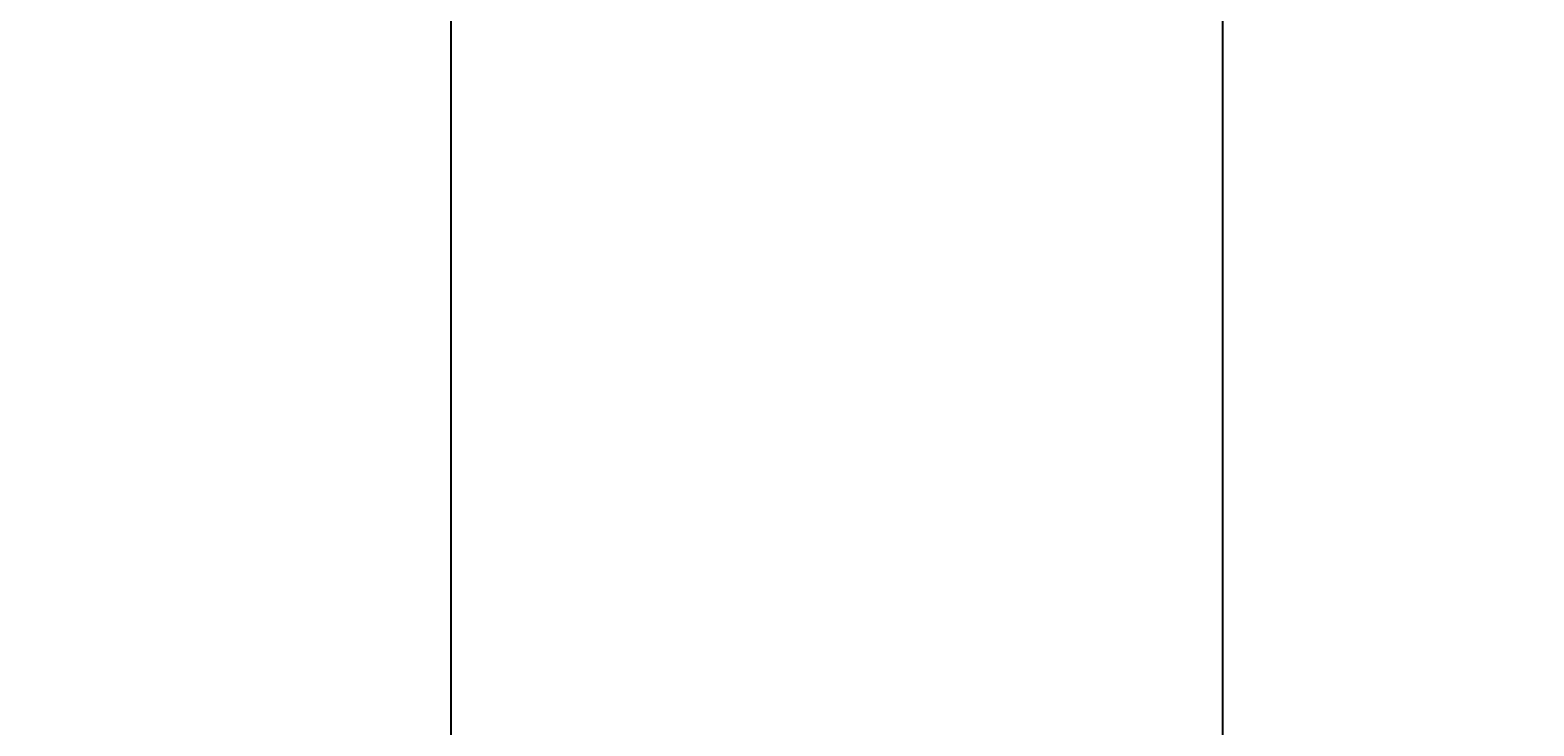
# Model space of a CAD drawing. Units: inches. Extents: x 35362 to 73946, y 43607 to 67532.
# Tile 47 of 134: x 47763 to 48533, y 46564 to 46919. Entities that reach past the tile are written whole.
import ezdxf

# ---------------------------------------------------------------- set-up
doc = ezdxf.new("R2010")
doc.units = ezdxf.units.IN
doc.header["$MEASUREMENT"] = 0
doc.layers.add('A-ANNO-DIMS', color=2, linetype='Continuous', lineweight=18)
doc.styles.get("Standard").update_dxf_attribs({"font": 'arial.ttf'})
doc.dimstyles.get("Standard").update_dxf_attribs({"dimtxt": 0.18, "dimasz": 0.18, "dimexe": 0.18, "dimexo": 0.0625, "dimgap": 0.09, "dimtad": 0, "dimtih": 1, "dimtoh": 1, "dimdec": 4, "dimzin": 0, "dimdsep": 46, "dimtxsty": 'Standard', "dimcen": 0.09, "dimadec": 0, "dimazin": 0, "dimtfac": 1, "dimtdec": 4, "dimtofl": 0, "dimtmove": 0, "dimatfit": 3, "dimfxl": 1, "dimtolj": 1, "dimtzin": 0, "dimarcsym": 0})

# ---------------------------------------------------------------- blocks, each defined once
blk = doc.blocks.new('*D5')
at = {"layer": 'A-ANNO-DIMS', "color": 0, "lineweight": -2, "transparency": 16777216}
for p, q in [((37121.95, 46919.32), (37121.95, 43606.68)), ((69871.5, 45449.83), (69871.5, 43606.68)), ((37122.13, 43606.86), (53496.29, 43606.86)), ((69871.32, 43606.86), (53497.15, 43606.86))]:
    blk.add_line(p, q, dxfattribs=at)
at = {"layer": 'A-ANNO-DIMS', "color": 0, "transparency": 16777216}
for points in [[(37122.13, 43606.89), (37122.13, 43606.83), (37121.95, 43606.86)], [(69871.32, 43606.89), (69871.32, 43606.83), (69871.5, 43606.86)]]:
    blk.add_solid(points, dxfattribs=at)
at = {"layer": 'Defpoints', "color": 0, "transparency": 16777216}
for p in [(37121.95, 46919.38), (69871.5, 45449.89), (69871.5, 43606.86)]:
    blk.add_point(p, dxfattribs=at)
at = {"layer": 'A-ANNO-DIMS', "color": 0, "transparency": 16777216, "insert": (53496.72, 43606.86), "char_height": 0.18, "attachment_point": 5}
blk.add_mtext('\\A1;32750', dxfattribs=at)
blk = doc.blocks.new('*D11')
at = {"layer": 'A-ANNO-DIMS', "color": 0, "lineweight": -2, "transparency": 16777216}
for p, q in [((47978.66, 56028.77), (47978.66, 43606.68)), ((53109.76, 56028.77), (53109.76, 43606.68)), ((47978.84, 43606.86), (50543.87, 43606.86)), ((53109.58, 43606.86), (50544.55, 43606.86))]:
    blk.add_line(p, q, dxfattribs=at)
at = {"layer": 'A-ANNO-DIMS', "color": 0, "transparency": 16777216}
for points in [[(47978.84, 43606.89), (47978.84, 43606.83), (47978.66, 43606.86)], [(53109.58, 43606.89), (53109.58, 43606.83), (53109.76, 43606.86)]]:
    blk.add_solid(points, dxfattribs=at)
at = {"layer": 'Defpoints', "color": 0, "transparency": 16777216}
for p in [(47978.66, 56028.84), (53109.76, 56028.84), (53109.76, 43606.86)]:
    blk.add_point(p, dxfattribs=at)
at = {"layer": 'A-ANNO-DIMS', "color": 0, "transparency": 16777216, "insert": (50544.21, 43606.86), "char_height": 0.18, "attachment_point": 5}
blk.add_mtext('\\A1;5131', dxfattribs=at)
blk = doc.blocks.new('*D13')
at = {"layer": 'A-ANNO-DIMS', "color": 0, "lineweight": -2, "transparency": 16777216}
for p, q in [((48373.49, 51694.02), (48373.49, 43606.68)), ((51029.04, 51694.02), (51029.04, 43606.68)), ((48373.67, 43606.86), (49700.8, 43606.86)), ((51028.86, 43606.86), (49701.73, 43606.86))]:
    blk.add_line(p, q, dxfattribs=at)
at = {"layer": 'A-ANNO-DIMS', "color": 0, "transparency": 16777216}
for points in [[(48373.67, 43606.89), (48373.67, 43606.83), (48373.49, 43606.86)], [(51028.86, 43606.89), (51028.86, 43606.83), (51029.04, 43606.86)]]:
    blk.add_solid(points, dxfattribs=at)
at = {"layer": 'Defpoints', "color": 0, "transparency": 16777216}
for p in [(48373.49, 51694.09), (51029.04, 51694.09), (51029.04, 43606.86)]:
    blk.add_point(p, dxfattribs=at)
at = {"layer": 'A-ANNO-DIMS', "color": 0, "transparency": 16777216, "insert": (49701.27, 43606.86), "char_height": 0.18, "attachment_point": 5}
blk.add_mtext('\\A1;2655.6', dxfattribs=at)
blk = doc.blocks.new('*D27')
at = {"layer": 'A-ANNO-DIMS', "color": 0, "lineweight": -2, "transparency": 16777216}
for p, q in [((47978.66, 56028.77), (47978.66, 43606.68)), ((48373.49, 53428.96), (48373.49, 43606.68)), ((47978.84, 43606.86), (48175.68, 43606.86)), ((48373.31, 43606.86), (48176.47, 43606.86))]:
    blk.add_line(p, q, dxfattribs=at)
at = {"layer": 'A-ANNO-DIMS', "color": 0, "transparency": 16777216}
for points in [[(47978.84, 43606.89), (47978.84, 43606.83), (47978.66, 43606.86)], [(48373.31, 43606.89), (48373.31, 43606.83), (48373.49, 43606.86)]]:
    blk.add_solid(points, dxfattribs=at)
at = {"layer": 'Defpoints', "color": 0, "transparency": 16777216}
for p in [(47978.66, 56028.84), (48373.49, 53429.02), (48373.49, 43606.86)]:
    blk.add_point(p, dxfattribs=at)
at = {"layer": 'A-ANNO-DIMS', "color": 0, "transparency": 16777216, "insert": (48176.08, 43606.86), "char_height": 0.18, "attachment_point": 5}
blk.add_mtext('\\A1;394.8', dxfattribs=at)
blk = doc.blocks.new('*D67')
at = {"layer": 'A-ANNO-DIMS', "color": 0, "lineweight": -2, "transparency": 16777216}
for p, q in [((56873.54, 53351.53), (35361.77, 53351.53)), ((35361.95, 53351.35), (35361.95, 49400.89)), ((35361.95, 45450.07), (35361.95, 49400.53)), ((53793.58, 45449.89), (35361.77, 45449.89))]:
    blk.add_line(p, q, dxfattribs=at)
at = {"layer": 'A-ANNO-DIMS', "color": 0, "transparency": 16777216}
for points in [[(35361.92, 53351.35), (35361.98, 53351.35), (35361.95, 53351.53)], [(35361.92, 45450.07), (35361.98, 45450.07), (35361.95, 45449.89)]]:
    blk.add_solid(points, dxfattribs=at)
at = {"layer": 'Defpoints', "color": 0, "transparency": 16777216}
for p in [(35361.95, 53351.53), (56873.6, 53351.53), (53793.64, 45449.89)]:
    blk.add_point(p, dxfattribs=at)
at = {"layer": 'A-ANNO-DIMS', "color": 0, "transparency": 16777216, "insert": (35361.95, 49400.71), "char_height": 0.18, "attachment_point": 5}
blk.add_mtext('\\A1;7901.6', dxfattribs=at)
blk = doc.blocks.new('*D90')
at = {"layer": 'A-ANNO-DIMS', "color": 0, "lineweight": -2, "transparency": 16777216}
for p, q in [((53707.72, 47291.29), (35361.77, 47291.29)), ((35361.95, 47291.11), (35361.95, 46710.26)), ((35361.95, 46129.06), (35361.95, 46709.9)), ((53793.58, 46128.88), (35361.77, 46128.88))]:
    blk.add_line(p, q, dxfattribs=at)
at = {"layer": 'A-ANNO-DIMS', "color": 0, "transparency": 16777216}
for points in [[(35361.92, 47291.11), (35361.98, 47291.11), (35361.95, 47291.29)], [(35361.92, 46129.06), (35361.98, 46129.06), (35361.95, 46128.88)]]:
    blk.add_solid(points, dxfattribs=at)
at = {"layer": 'Defpoints', "color": 0, "transparency": 16777216}
for p in [(53707.78, 47291.29), (35361.95, 46128.88), (53793.64, 46128.88)]:
    blk.add_point(p, dxfattribs=at)
at = {"layer": 'A-ANNO-DIMS', "color": 0, "transparency": 16777216, "insert": (35361.95, 46710.08), "char_height": 0.18, "attachment_point": 5}
blk.add_mtext('\\A1;1162.4', dxfattribs=at)

msp = doc.modelspace()

# ---------------------------------------------------------------- dimensions: what is measured, and where the dimension line sits
at = {"layer": 'A-ANNO-DIMS'}
for base, p1, p2, override, picture, middle in [((53109.76, 43606.859), (47978.665, 56028.836), (53109.76, 56028.836), {"dimdec": 0, "dimlfac": 1, "dimrnd": 0, "dimzin": 0, "dimdsep": 46, "dimlunit": 2}, '*D11', (50544.212, 43606.859)), ((48373.492, 43606.859), (47978.665, 56028.836), (48373.492, 53429.019), {"dimdec": 1, "dimlfac": 1, "dimrnd": 0, "dimzin": 0, "dimdsep": 46, "dimlunit": 2}, '*D27', (48176.078, 43606.859)), ((51029.043, 43606.859), (48373.492, 51694.087), (51029.043, 51694.087), {"dimdec": 1, "dimlfac": 1, "dimrnd": 0, "dimzin": 0, "dimdsep": 46, "dimlunit": 2}, '*D13', (49701.267, 43606.859)), ((69871.496, 43606.859), (37121.949, 46919.381), (69871.496, 45449.894), {"dimdec": 0, "dimlfac": 1, "dimrnd": 0, "dimzin": 0, "dimdsep": 46, "dimlunit": 2}, '*D5', (53496.723, 43606.859))]:
    dim = msp.add_linear_dim(base=base, p1=p1, p2=p2, dimstyle='Standard', override=override, dxfattribs=at)
    dim.commit()
    dim.dimension.update_dxf_attribs({"geometry": picture, "text_midpoint": middle})
for base, p1, p2, picture, middle in [((35361.949, 53351.529), (53793.638, 45449.894), (56873.602, 53351.529), '*D67', (35361.949, 49400.712)), ((35361.949, 46128.878), (53707.781, 47291.285), (53793.638, 46128.878), '*D90', (35361.949, 46710.081))]:
    dim = msp.add_linear_dim(base=base, p1=p1, p2=p2, angle=90, dimstyle='Standard', override={"dimdec": 1, "dimlfac": 1, "dimrnd": 0, "dimzin": 0, "dimdsep": 46, "dimlunit": 2}, dxfattribs=at)
    dim.commit()
    dim.dimension.update_dxf_attribs({"geometry": picture, "text_midpoint": middle})

doc.saveas('drawing.dxf')
